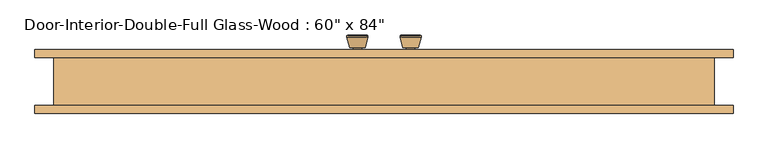
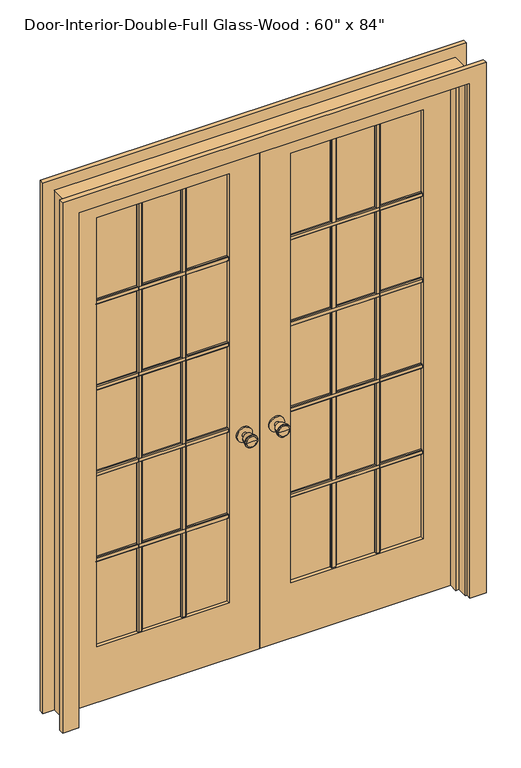
"""IFC4 building model written with IfcOpenShell, lengths in millimetres: door geometry."""

from ifc_helpers import new_model, si_unit, point, frame, frame_2d, origin, place, context, project, spatial, polyline, circle_curve, trimmed, segment, composite_curve, outline, extrude, faceted_brep, source, transform, mapped, element, save
from ifc_brep_helpers import plane_surface, cylinder_surface, revolved_surface, advanced_brep


def door_fac3bb52(model_context):
    return source(origin(), model_context, "Body", "SolidModel", [
        advanced_brep(
        [(-63.5, 59.975, 914.4), (-73.5, 59.975, 914.4), (-53.5, 59.975, 914.4), (-83.9758676, 108.975, 914.4), (-63.5, 108.975, 914.4), (-43.0241324, 108.975, 914.4), (-88.5, 107.1471319, 914.4), (-38.5, 107.1471319, 914.4), (-88.5, 103.6834537, 914.4), (-38.5, 103.6834537, 914.4), (-82.136236, 78.975, 914.4), (-44.863764, 78.975, 914.4), (-73.5, 78.975, 914.4), (-53.5, 78.975, 914.4)],
        [
            (0, 1),
            (1, 2, circle_curve(frame((-63.5, 59.975, 914.4), z_axis=(0.0, -1.0, 0.0), x_axis=(1.0, 0.0, 0.0)), 10.0)),
            (2, 0),
            (2, 1, circle_curve(frame((-63.5, 59.975, 914.4), z_axis=(0.0, -1.0, 0.0), x_axis=(1.0, 0.0, 0.0)), 10.0)),
            (3, 4),
            (4, 5),
            (5, 3, circle_curve(frame((-63.5, 108.975, 914.4), z_axis=(0.0, 1.0, 0.0), x_axis=(1.0, 0.0, 0.0)), 20.4758676)),
            (3, 5, circle_curve(frame((-63.5, 108.975, 914.4), z_axis=(0.0, 1.0, 0.0), x_axis=(1.0, 0.0, 0.0)), 20.4758676)),
            (6, 3),
            (5, 7),
            (7, 6, circle_curve(frame((-63.5, 107.1471319, 914.4), z_axis=(0.0, 1.0, 0.0), x_axis=(1.0, 0.0, 0.0)), 25.0)),
            (6, 7, circle_curve(frame((-63.5, 107.1471319, 914.4), z_axis=(0.0, 1.0, 0.0), x_axis=(1.0, 0.0, 0.0)), 25.0)),
            (8, 6),
            (7, 9),
            (9, 8, circle_curve(frame((-63.5, 103.6834537, 914.4), z_axis=(0.0, 1.0, 0.0), x_axis=(1.0, 0.0, 0.0)), 25.0)),
            (8, 9, circle_curve(frame((-63.5, 103.6834537, 914.4), z_axis=(0.0, 1.0, 0.0), x_axis=(1.0, 0.0, 0.0)), 25.0)),
            (10, 8),
            (9, 11),
            (11, 10, circle_curve(frame((-63.5, 78.975, 914.4), z_axis=(0.0, 1.0, 0.0), x_axis=(1.0, 0.0, 0.0)), 18.636236)),
            (10, 11, circle_curve(frame((-63.5, 78.975, 914.4), z_axis=(0.0, 1.0, 0.0), x_axis=(1.0, 0.0, 0.0)), 18.636236)),
            (12, 10),
            (11, 13),
            (13, 12, circle_curve(frame((-63.5, 78.975, 914.4), z_axis=(0.0, 1.0, 0.0), x_axis=(1.0, 0.0, 0.0)), 10.0)),
            (12, 13, circle_curve(frame((-63.5, 78.975, 914.4), z_axis=(0.0, 1.0, 0.0), x_axis=(1.0, 0.0, 0.0)), 10.0)),
            (1, 12),
            (13, 2),
        ],
        [
            plane_surface(frame((-63.5, 59.975, 914.4), z_axis=(0.0, -1.0, 0.0), x_axis=(1.0, 0.0, 0.0))),
            plane_surface(frame((-63.5, 108.975, 914.4), z_axis=(0.0, 1.0, 0.0), x_axis=(1.0, 0.0, 0.0))),
            revolved_surface(polyline([(-43.0241324, 108.975, 914.4), (-38.5, 107.1471319, 914.4)]), (-63.5, 59.975, 914.4), (0.0, -1.0, 0.0)),
            cylinder_surface(frame((-63.5, 59.975, 914.4), z_axis=(0.0, -1.0, 0.0), x_axis=(1.0, 0.0, 0.0)), 25.0),
            revolved_surface(polyline([(-38.5, 103.6834537, 914.4), (-44.863764, 78.975, 914.4)]), (-63.5, 59.975, 914.4), (0.0, -1.0, 0.0)),
            plane_surface(frame((-63.5, 78.975, 914.4), z_axis=(0.0, -1.0, 0.0), x_axis=(1.0, 0.0, 0.0))),
            cylinder_surface(frame((-63.5, 59.975, 914.4), z_axis=(0.0, -1.0, 0.0), x_axis=(1.0, 0.0, 0.0)), 10.0),
        ],
        [
            (0, [[1, 2, 3]]),
            (0, [[-3, 4, -1]]),
            (1, [[5, 6, 7]]),
            (1, [[-6, -5, 8]]),
            (2, [[9, -7, 10, 11]]),
            (2, [[-10, -8, -9, 12]]),
            (3, [[13, -11, 14, 15]]),
            (3, [[-14, -12, -13, 16]]),
            (4, [[17, -15, 18, 19]]),
            (4, [[-18, -16, -17, 20]]),
            (5, [[21, -19, 22, 23]]),
            (5, [[-22, -20, -21, 24]]),
            (6, [[25, -23, 26, -2]]),
            (6, [[-26, -24, -25, -4]]),
        ],
    ),
        extrude(outline(composite_curve([segment(trimmed(circle_curve(frame_2d((914.4, -63.5)), 30.0), [point((914.4, -33.5))], [point((914.4, -93.5))], False, "CARTESIAN"), True, "CONTINUOUS"), segment(trimmed(circle_curve(frame_2d((914.4, -63.5)), 30.0), [point((914.4, -93.5))], [point((914.4, -33.5))], False, "CARTESIAN"), True, "CONTINUOUS")], self_intersect=False)), frame((0.0, 53.975, 0.0), z_axis=(0.0, 1.0, 0.0), x_axis=(0.0, 0.0, 1.0)), (0.0, 0.0, 1.0), 6.0),
        advanced_brep(
        [(-63.5, 13.05, 914.4), (-53.5, 13.05, 914.4), (-73.5, 13.05, 914.4), (-83.9758676, -35.95, 914.4), (-43.0241324, -35.95, 914.4), (-63.5, -35.95, 914.4), (-88.5, -34.1221319, 914.4), (-38.5, -34.1221319, 914.4), (-88.5, -30.6584537, 914.4), (-38.5, -30.6584537, 914.4), (-82.136236, -5.95, 914.4), (-44.863764, -5.95, 914.4), (-73.5, -5.95, 914.4), (-53.5, -5.95, 914.4)],
        [
            (0, 1),
            (1, 2, circle_curve(frame((-63.5, 13.05, 914.4), z_axis=(0.0, 1.0, 0.0), x_axis=(1.0, 0.0, 0.0)), 10.0)),
            (2, 0),
            (2, 1, circle_curve(frame((-63.5, 13.05, 914.4), z_axis=(0.0, 1.0, 0.0), x_axis=(1.0, 0.0, 0.0)), 10.0)),
            (3, 4, circle_curve(frame((-63.5, -35.95, 914.4), z_axis=(0.0, -1.0, 0.0), x_axis=(1.0, 0.0, 0.0)), 20.4758676)),
            (4, 5),
            (5, 3),
            (4, 3, circle_curve(frame((-63.5, -35.95, 914.4), z_axis=(0.0, -1.0, 0.0), x_axis=(1.0, 0.0, 0.0)), 20.4758676)),
            (6, 7, circle_curve(frame((-63.5, -34.1221319, 914.4), z_axis=(0.0, -1.0, 0.0), x_axis=(1.0, 0.0, 0.0)), 25.0)),
            (7, 4),
            (3, 6),
            (7, 6, circle_curve(frame((-63.5, -34.1221319, 914.4), z_axis=(0.0, -1.0, 0.0), x_axis=(1.0, 0.0, 0.0)), 25.0)),
            (8, 9, circle_curve(frame((-63.5, -30.6584537, 914.4), z_axis=(0.0, -1.0, 0.0), x_axis=(1.0, 0.0, 0.0)), 25.0)),
            (9, 7),
            (6, 8),
            (9, 8, circle_curve(frame((-63.5, -30.6584537, 914.4), z_axis=(0.0, -1.0, 0.0), x_axis=(1.0, 0.0, 0.0)), 25.0)),
            (10, 11, circle_curve(frame((-63.5, -5.95, 914.4), z_axis=(0.0, -1.0, 0.0), x_axis=(1.0, 0.0, 0.0)), 18.636236)),
            (11, 9),
            (8, 10),
            (11, 10, circle_curve(frame((-63.5, -5.95, 914.4), z_axis=(0.0, -1.0, 0.0), x_axis=(1.0, 0.0, 0.0)), 18.636236)),
            (12, 13, circle_curve(frame((-63.5, -5.95, 914.4), z_axis=(0.0, -1.0, 0.0), x_axis=(1.0, 0.0, 0.0)), 10.0)),
            (13, 11),
            (10, 12),
            (13, 12, circle_curve(frame((-63.5, -5.95, 914.4), z_axis=(0.0, -1.0, 0.0), x_axis=(1.0, 0.0, 0.0)), 10.0)),
            (1, 13),
            (12, 2),
        ],
        [
            plane_surface(frame((-63.5, 13.05, 914.4), z_axis=(0.0, 1.0, 0.0), x_axis=(1.0, 0.0, 0.0))),
            plane_surface(frame((-63.5, -35.95, 914.4), z_axis=(0.0, -1.0, 0.0), x_axis=(1.0, 0.0, 0.0))),
            revolved_surface(polyline([(-43.0241324, -35.95, 914.4), (-38.5, -34.1221319, 914.4)]), (-63.5, 13.05, 914.4), (0.0, 1.0, 0.0)),
            cylinder_surface(frame((-63.5, 13.05, 914.4), z_axis=(0.0, 1.0, 0.0), x_axis=(1.0, 0.0, 0.0)), 25.0),
            revolved_surface(polyline([(-38.5, -30.6584537, 914.4), (-44.863764, -5.95, 914.4)]), (-63.5, 13.05, 914.4), (0.0, 1.0, 0.0)),
            plane_surface(frame((-63.5, -5.95, 914.4), z_axis=(0.0, 1.0, 0.0), x_axis=(1.0, 0.0, 0.0))),
            cylinder_surface(frame((-63.5, 13.05, 914.4), z_axis=(0.0, 1.0, 0.0), x_axis=(1.0, 0.0, 0.0)), 10.0),
        ],
        [
            (0, [[1, 2, 3]]),
            (0, [[-3, 4, -1]]),
            (1, [[5, 6, 7]]),
            (1, [[8, -7, -6]]),
            (2, [[9, 10, -5, 11]]),
            (2, [[12, -11, -8, -10]]),
            (3, [[13, 14, -9, 15]]),
            (3, [[16, -15, -12, -14]]),
            (4, [[17, 18, -13, 19]]),
            (4, [[20, -19, -16, -18]]),
            (5, [[21, 22, -17, 23]]),
            (5, [[24, -23, -20, -22]]),
            (6, [[-2, 25, -21, 26]]),
            (6, [[-4, -26, -24, -25]]),
        ],
    ),
        extrude(outline(composite_curve([segment(trimmed(circle_curve(frame_2d((914.4, -63.5)), 30.0), [point((914.4, -33.5))], [point((914.4, -93.5))], False, "CARTESIAN"), True, "CONTINUOUS"), segment(trimmed(circle_curve(frame_2d((914.4, -63.5)), 30.0), [point((914.4, -93.5))], [point((914.4, -33.5))], False, "CARTESIAN"), True, "CONTINUOUS")], self_intersect=False)), frame((0.0, 13.05, 0.0), z_axis=(0.0, 1.0, 0.0), x_axis=(0.0, 0.0, 1.0)), (0.0, 0.0, 1.0), 6.0),
        extrude(outline(polyline([(33.02, 1667.51), (33.02, 1648.46), (26.67, 1648.46), (23.495, 1651.635), (23.495, 1664.335), (26.67, 1667.51), (33.02, 1667.51)])), frame((120.65, 0.0, 0.0), z_axis=(1.0, 0.0, 0.0), x_axis=(0.0, 1.0, 0.0)), (0.0, 0.0, 1.0), 520.7),
        extrude(outline(polyline([(33.02, 1310.9575), (33.02, 1291.9075), (26.67, 1291.9075), (23.495, 1295.0825), (23.495, 1307.7825), (26.67, 1310.9575), (33.02, 1310.9575)])), frame((120.65, 0.0, 0.0), z_axis=(1.0, 0.0, 0.0), x_axis=(0.0, 1.0, 0.0)), (0.0, 0.0, 1.0), 520.7),
        extrude(outline(polyline([(33.02, 954.405), (33.02, 935.355), (26.67, 935.355), (23.495, 938.53), (23.495, 951.23), (26.67, 954.405), (33.02, 954.405)])), frame((120.65, 0.0, 0.0), z_axis=(1.0, 0.0, 0.0), x_axis=(0.0, 1.0, 0.0)), (0.0, 0.0, 1.0), 520.7),
        extrude(outline(polyline([(33.02, 597.8525), (33.02, 578.8025), (26.67, 578.8025), (23.495, 581.9775), (23.495, 594.6775), (26.67, 597.8525), (33.02, 597.8525)])), frame((120.65, 0.0, 0.0), z_axis=(1.0, 0.0, 0.0), x_axis=(0.0, 1.0, 0.0)), (0.0, 0.0, 1.0), 520.7),
        extrude(outline(polyline([(458.2583333, 33.02), (477.3083333, 33.02), (477.3083333, 26.67), (474.1333333, 23.495), (461.4333333, 23.495), (458.2583333, 26.67), (458.2583333, 33.02)])), frame((0.0, 0.0, 231.775), z_axis=(0.0, 0.0, 1.0), x_axis=(1.0, 0.0, 0.0)), (0.0, 0.0, 1.0), 1782.7625),
        extrude(outline(polyline([(284.6916667, 33.02), (303.7416667, 33.02), (303.7416667, 26.67), (300.5666667, 23.495), (287.8666667, 23.495), (284.6916667, 26.67), (284.6916667, 33.02)])), frame((0.0, 0.0, 231.775), z_axis=(0.0, 0.0, 1.0), x_axis=(1.0, 0.0, 0.0)), (0.0, 0.0, 1.0), 1782.7625),
        extrude(outline(polyline([(40.005, 1667.51), (46.355, 1667.51), (49.53, 1664.335), (49.53, 1651.635), (46.355, 1648.46), (40.005, 1648.46), (40.005, 1667.51)])), frame((-641.35, 0.0, 0.0), z_axis=(1.0, 0.0, 0.0), x_axis=(0.0, 1.0, 0.0)), (0.0, 0.0, 1.0), 520.7),
        extrude(outline(polyline([(40.005, 1310.9575), (46.355, 1310.9575), (49.53, 1307.7825), (49.53, 1295.0825), (46.355, 1291.9075), (40.005, 1291.9075), (40.005, 1310.9575)])), frame((-641.35, 0.0, 0.0), z_axis=(1.0, 0.0, 0.0), x_axis=(0.0, 1.0, 0.0)), (0.0, 0.0, 1.0), 520.7),
        extrude(outline(polyline([(40.005, 954.405), (46.355, 954.405), (49.53, 951.23), (49.53, 938.53), (46.355, 935.355), (40.005, 935.355), (40.005, 954.405)])), frame((-641.35, 0.0, 0.0), z_axis=(1.0, 0.0, 0.0), x_axis=(0.0, 1.0, 0.0)), (0.0, 0.0, 1.0), 520.7),
        extrude(outline(polyline([(40.005, 597.8525), (46.355, 597.8525), (49.53, 594.6775), (49.53, 581.9775), (46.355, 578.8025), (40.005, 578.8025), (40.005, 597.8525)])), frame((-641.35, 0.0, 0.0), z_axis=(1.0, 0.0, 0.0), x_axis=(0.0, 1.0, 0.0)), (0.0, 0.0, 1.0), 520.7),
        extrude(outline(polyline([(-303.7416667, 40.005), (-303.7416667, 46.355), (-300.5666667, 49.53), (-287.8666667, 49.53), (-284.6916667, 46.355), (-284.6916667, 40.005), (-303.7416667, 40.005)])), frame((0.0, 0.0, 231.775), z_axis=(0.0, 0.0, 1.0), x_axis=(1.0, 0.0, 0.0)), (0.0, 0.0, 1.0), 1782.7625),
        extrude(outline(polyline([(-477.3083333, 40.005), (-477.3083333, 46.355), (-474.1333333, 49.53), (-461.4333333, 49.53), (-458.2583333, 46.355), (-458.2583333, 40.005), (-477.3083333, 40.005)])), frame((0.0, 0.0, 231.775), z_axis=(0.0, 0.0, 1.0), x_axis=(1.0, 0.0, 0.0)), (0.0, 0.0, 1.0), 1782.7625),
        extrude(outline(polyline([(40.005, 1667.51), (46.355, 1667.51), (49.53, 1664.335), (49.53, 1651.635), (46.355, 1648.46), (40.005, 1648.46), (40.005, 1667.51)])), frame((120.65, 0.0, 0.0), z_axis=(1.0, 0.0, 0.0), x_axis=(0.0, 1.0, 0.0)), (0.0, 0.0, 1.0), 520.7),
        extrude(outline(polyline([(40.005, 1310.9575), (46.355, 1310.9575), (49.53, 1307.7825), (49.53, 1295.0825), (46.355, 1291.9075), (40.005, 1291.9075), (40.005, 1310.9575)])), frame((120.65, 0.0, 0.0), z_axis=(1.0, 0.0, 0.0), x_axis=(0.0, 1.0, 0.0)), (0.0, 0.0, 1.0), 520.7),
        extrude(outline(polyline([(40.005, 954.405), (46.355, 954.405), (49.53, 951.23), (49.53, 938.53), (46.355, 935.355), (40.005, 935.355), (40.005, 954.405)])), frame((120.65, 0.0, 0.0), z_axis=(1.0, 0.0, 0.0), x_axis=(0.0, 1.0, 0.0)), (0.0, 0.0, 1.0), 520.7),
        extrude(outline(polyline([(40.005, 597.8525), (46.355, 597.8525), (49.53, 594.6775), (49.53, 581.9775), (46.355, 578.8025), (40.005, 578.8025), (40.005, 597.8525)])), frame((120.65, 0.0, 0.0), z_axis=(1.0, 0.0, 0.0), x_axis=(0.0, 1.0, 0.0)), (0.0, 0.0, 1.0), 520.7),
        extrude(outline(polyline([(458.2583333, 40.005), (458.2583333, 46.355), (461.4333333, 49.53), (474.1333333, 49.53), (477.3083333, 46.355), (477.3083333, 40.005), (458.2583333, 40.005)])), frame((0.0, 0.0, 231.775), z_axis=(0.0, 0.0, 1.0), x_axis=(1.0, 0.0, 0.0)), (0.0, 0.0, 1.0), 1782.7625),
        extrude(outline(polyline([(284.6916667, 40.005), (284.6916667, 46.355), (287.8666667, 49.53), (300.5666667, 49.53), (303.7416667, 46.355), (303.7416667, 40.005), (284.6916667, 40.005)])), frame((0.0, 0.0, 231.775), z_axis=(0.0, 0.0, 1.0), x_axis=(1.0, 0.0, 0.0)), (0.0, 0.0, 1.0), 1782.7625),
        extrude(outline(polyline([(33.02, 1667.51), (33.02, 1648.46), (26.67, 1648.46), (23.495, 1651.635), (23.495, 1664.335), (26.67, 1667.51), (33.02, 1667.51)])), frame((-641.35, 0.0, 0.0), z_axis=(1.0, 0.0, 0.0), x_axis=(0.0, 1.0, 0.0)), (0.0, 0.0, 1.0), 520.7),
        extrude(outline(polyline([(33.02, 1310.9575), (33.02, 1291.9075), (26.67, 1291.9075), (23.495, 1295.0825), (23.495, 1307.7825), (26.67, 1310.9575), (33.02, 1310.9575)])), frame((-641.35, 0.0, 0.0), z_axis=(1.0, 0.0, 0.0), x_axis=(0.0, 1.0, 0.0)), (0.0, 0.0, 1.0), 520.7),
        extrude(outline(polyline([(33.02, 954.405), (33.02, 935.355), (26.67, 935.355), (23.495, 938.53), (23.495, 951.23), (26.67, 954.405), (33.02, 954.405)])), frame((-641.35, 0.0, 0.0), z_axis=(1.0, 0.0, 0.0), x_axis=(0.0, 1.0, 0.0)), (0.0, 0.0, 1.0), 520.7),
        extrude(outline(polyline([(33.02, 597.8525), (33.02, 578.8025), (26.67, 578.8025), (23.495, 581.9775), (23.495, 594.6775), (26.67, 597.8525), (33.02, 597.8525)])), frame((-641.35, 0.0, 0.0), z_axis=(1.0, 0.0, 0.0), x_axis=(0.0, 1.0, 0.0)), (0.0, 0.0, 1.0), 520.7),
        extrude(outline(polyline([(-303.7416667, 33.02), (-284.6916667, 33.02), (-284.6916667, 26.67), (-287.8666667, 23.495), (-300.5666667, 23.495), (-303.7416667, 26.67), (-303.7416667, 33.02)])), frame((0.0, 0.0, 231.775), z_axis=(0.0, 0.0, 1.0), x_axis=(1.0, 0.0, 0.0)), (0.0, 0.0, 1.0), 1782.7625),
        extrude(outline(polyline([(-477.3083333, 33.02), (-458.2583333, 33.02), (-458.2583333, 26.67), (-461.4333333, 23.495), (-474.1333333, 23.495), (-477.3083333, 26.67), (-477.3083333, 33.02)])), frame((0.0, 0.0, 231.775), z_axis=(0.0, 0.0, 1.0), x_axis=(1.0, 0.0, 0.0)), (0.0, 0.0, 1.0), 1782.7625),
        advanced_brep(
        [(63.5, 13.05, 914.4), (73.5, 13.05, 914.4), (53.5, 13.05, 914.4), (83.9758676, -35.95, 914.4), (63.5, -35.95, 914.4), (43.0241324, -35.95, 914.4), (88.5, -34.1221319, 914.4), (38.5, -34.1221319, 914.4), (88.5, -30.6584537, 914.4), (38.5, -30.6584537, 914.4), (82.136236, -5.95, 914.4), (44.863764, -5.95, 914.4), (73.5, -5.95, 914.4), (53.5, -5.95, 914.4)],
        [
            (0, 1),
            (1, 2, circle_curve(frame((63.5, 13.05, 914.4), z_axis=(0.0, 1.0, 0.0), x_axis=(-1.0, 0.0, 0.0)), 10.0)),
            (2, 0),
            (2, 1, circle_curve(frame((63.5, 13.05, 914.4), z_axis=(0.0, 1.0, 0.0), x_axis=(-1.0, 0.0, 0.0)), 10.0)),
            (3, 4),
            (4, 5),
            (5, 3, circle_curve(frame((63.5, -35.95, 914.4), z_axis=(0.0, -1.0, 0.0), x_axis=(-1.0, 0.0, 0.0)), 20.4758676)),
            (3, 5, circle_curve(frame((63.5, -35.95, 914.4), z_axis=(0.0, -1.0, 0.0), x_axis=(-1.0, 0.0, 0.0)), 20.4758676)),
            (6, 3),
            (5, 7),
            (7, 6, circle_curve(frame((63.5, -34.1221319, 914.4), z_axis=(0.0, -1.0, 0.0), x_axis=(-1.0, 0.0, 0.0)), 25.0)),
            (6, 7, circle_curve(frame((63.5, -34.1221319, 914.4), z_axis=(0.0, -1.0, 0.0), x_axis=(-1.0, 0.0, 0.0)), 25.0)),
            (8, 6),
            (7, 9),
            (9, 8, circle_curve(frame((63.5, -30.6584537, 914.4), z_axis=(0.0, -1.0, 0.0), x_axis=(-1.0, 0.0, 0.0)), 25.0)),
            (8, 9, circle_curve(frame((63.5, -30.6584537, 914.4), z_axis=(0.0, -1.0, 0.0), x_axis=(-1.0, 0.0, 0.0)), 25.0)),
            (10, 8),
            (9, 11),
            (11, 10, circle_curve(frame((63.5, -5.95, 914.4), z_axis=(0.0, -1.0, 0.0), x_axis=(-1.0, 0.0, 0.0)), 18.636236)),
            (10, 11, circle_curve(frame((63.5, -5.95, 914.4), z_axis=(0.0, -1.0, 0.0), x_axis=(-1.0, 0.0, 0.0)), 18.636236)),
            (12, 10),
            (11, 13),
            (13, 12, circle_curve(frame((63.5, -5.95, 914.4), z_axis=(0.0, -1.0, 0.0), x_axis=(-1.0, 0.0, 0.0)), 10.0)),
            (12, 13, circle_curve(frame((63.5, -5.95, 914.4), z_axis=(0.0, -1.0, 0.0), x_axis=(-1.0, 0.0, 0.0)), 10.0)),
            (1, 12),
            (13, 2),
        ],
        [
            plane_surface(frame((63.5, 13.05, 914.4), z_axis=(0.0, 1.0, 0.0), x_axis=(-1.0, 0.0, 0.0))),
            plane_surface(frame((63.5, -35.95, 914.4), z_axis=(0.0, -1.0, 0.0), x_axis=(-1.0, 0.0, 0.0))),
            revolved_surface(polyline([(43.0241324, -35.95, 914.4), (38.5, -34.1221319, 914.4)]), (63.5, 13.05, 914.4), (0.0, 1.0, 0.0)),
            cylinder_surface(frame((63.5, 13.05, 914.4), z_axis=(0.0, 1.0, 0.0), x_axis=(-1.0, 0.0, 0.0)), 25.0),
            revolved_surface(polyline([(38.5, -30.6584537, 914.4), (44.863764, -5.95, 914.4)]), (63.5, 13.05, 914.4), (0.0, 1.0, 0.0)),
            plane_surface(frame((63.5, -5.95, 914.4), z_axis=(0.0, 1.0, 0.0), x_axis=(-1.0, 0.0, 0.0))),
            cylinder_surface(frame((63.5, 13.05, 914.4), z_axis=(0.0, 1.0, 0.0), x_axis=(-1.0, 0.0, 0.0)), 10.0),
        ],
        [
            (0, [[1, 2, 3]]),
            (0, [[-3, 4, -1]]),
            (1, [[5, 6, 7]]),
            (1, [[-6, -5, 8]]),
            (2, [[9, -7, 10, 11]]),
            (2, [[-10, -8, -9, 12]]),
            (3, [[13, -11, 14, 15]]),
            (3, [[-14, -12, -13, 16]]),
            (4, [[17, -15, 18, 19]]),
            (4, [[-18, -16, -17, 20]]),
            (5, [[21, -19, 22, 23]]),
            (5, [[-22, -20, -21, 24]]),
            (6, [[25, -23, 26, -2]]),
            (6, [[-26, -24, -25, -4]]),
        ],
    ),
        extrude(outline(composite_curve([segment(trimmed(circle_curve(frame_2d((914.4, 63.5)), 30.0), [point((914.4, 33.5))], [point((914.4, 93.5))], False, "CARTESIAN"), True, "CONTINUOUS"), segment(trimmed(circle_curve(frame_2d((914.4, 63.5)), 30.0), [point((914.4, 93.5))], [point((914.4, 33.5))], False, "CARTESIAN"), True, "CONTINUOUS")], self_intersect=False)), frame((0.0, 13.05, 0.0), z_axis=(0.0, 1.0, 0.0), x_axis=(0.0, 0.0, 1.0)), (0.0, 0.0, 1.0), 6.0),
        advanced_brep(
        [(63.5, 59.975, 914.4), (53.5, 59.975, 914.4), (73.5, 59.975, 914.4), (83.9758676, 108.975, 914.4), (43.0241324, 108.975, 914.4), (63.5, 108.975, 914.4), (88.5, 107.1471319, 914.4), (38.5, 107.1471319, 914.4), (88.5, 103.6834537, 914.4), (38.5, 103.6834537, 914.4), (82.136236, 78.975, 914.4), (44.863764, 78.975, 914.4), (73.5, 78.975, 914.4), (53.5, 78.975, 914.4)],
        [
            (0, 1),
            (1, 2, circle_curve(frame((63.5, 59.975, 914.4), z_axis=(0.0, -1.0, 0.0), x_axis=(-1.0, 0.0, 0.0)), 10.0)),
            (2, 0),
            (2, 1, circle_curve(frame((63.5, 59.975, 914.4), z_axis=(0.0, -1.0, 0.0), x_axis=(-1.0, 0.0, 0.0)), 10.0)),
            (3, 4, circle_curve(frame((63.5, 108.975, 914.4), z_axis=(0.0, 1.0, 0.0), x_axis=(-1.0, 0.0, 0.0)), 20.4758676)),
            (4, 5),
            (5, 3),
            (4, 3, circle_curve(frame((63.5, 108.975, 914.4), z_axis=(0.0, 1.0, 0.0), x_axis=(-1.0, 0.0, 0.0)), 20.4758676)),
            (6, 7, circle_curve(frame((63.5, 107.1471319, 914.4), z_axis=(0.0, 1.0, 0.0), x_axis=(-1.0, 0.0, 0.0)), 25.0)),
            (7, 4),
            (3, 6),
            (7, 6, circle_curve(frame((63.5, 107.1471319, 914.4), z_axis=(0.0, 1.0, 0.0), x_axis=(-1.0, 0.0, 0.0)), 25.0)),
            (8, 9, circle_curve(frame((63.5, 103.6834537, 914.4), z_axis=(0.0, 1.0, 0.0), x_axis=(-1.0, 0.0, 0.0)), 25.0)),
            (9, 7),
            (6, 8),
            (9, 8, circle_curve(frame((63.5, 103.6834537, 914.4), z_axis=(0.0, 1.0, 0.0), x_axis=(-1.0, 0.0, 0.0)), 25.0)),
            (10, 11, circle_curve(frame((63.5, 78.975, 914.4), z_axis=(0.0, 1.0, 0.0), x_axis=(-1.0, 0.0, 0.0)), 18.636236)),
            (11, 9),
            (8, 10),
            (11, 10, circle_curve(frame((63.5, 78.975, 914.4), z_axis=(0.0, 1.0, 0.0), x_axis=(-1.0, 0.0, 0.0)), 18.636236)),
            (12, 13, circle_curve(frame((63.5, 78.975, 914.4), z_axis=(0.0, 1.0, 0.0), x_axis=(-1.0, 0.0, 0.0)), 10.0)),
            (13, 11),
            (10, 12),
            (13, 12, circle_curve(frame((63.5, 78.975, 914.4), z_axis=(0.0, 1.0, 0.0), x_axis=(-1.0, 0.0, 0.0)), 10.0)),
            (1, 13),
            (12, 2),
        ],
        [
            plane_surface(frame((63.5, 59.975, 914.4), z_axis=(0.0, -1.0, 0.0), x_axis=(-1.0, 0.0, 0.0))),
            plane_surface(frame((63.5, 108.975, 914.4), z_axis=(0.0, 1.0, 0.0), x_axis=(-1.0, 0.0, 0.0))),
            revolved_surface(polyline([(43.0241324, 108.975, 914.4), (38.5, 107.1471319, 914.4)]), (63.5, 59.975, 914.4), (0.0, -1.0, 0.0)),
            cylinder_surface(frame((63.5, 59.975, 914.4), z_axis=(0.0, -1.0, 0.0), x_axis=(-1.0, 0.0, 0.0)), 25.0),
            revolved_surface(polyline([(38.5, 103.6834537, 914.4), (44.863764, 78.975, 914.4)]), (63.5, 59.975, 914.4), (0.0, -1.0, 0.0)),
            plane_surface(frame((63.5, 78.975, 914.4), z_axis=(0.0, -1.0, 0.0), x_axis=(-1.0, 0.0, 0.0))),
            cylinder_surface(frame((63.5, 59.975, 914.4), z_axis=(0.0, -1.0, 0.0), x_axis=(-1.0, 0.0, 0.0)), 10.0),
        ],
        [
            (0, [[1, 2, 3]]),
            (0, [[-3, 4, -1]]),
            (1, [[5, 6, 7]]),
            (1, [[8, -7, -6]]),
            (2, [[9, 10, -5, 11]]),
            (2, [[12, -11, -8, -10]]),
            (3, [[13, 14, -9, 15]]),
            (3, [[16, -15, -12, -14]]),
            (4, [[17, 18, -13, 19]]),
            (4, [[20, -19, -16, -18]]),
            (5, [[21, 22, -17, 23]]),
            (5, [[24, -23, -20, -22]]),
            (6, [[-2, 25, -21, 26]]),
            (6, [[-4, -26, -24, -25]]),
        ],
    ),
        extrude(outline(composite_curve([segment(trimmed(circle_curve(frame_2d((914.4, 63.5)), 30.0), [point((914.4, 33.5))], [point((914.4, 93.5))], False, "CARTESIAN"), True, "CONTINUOUS"), segment(trimmed(circle_curve(frame_2d((914.4, 63.5)), 30.0), [point((914.4, 93.5))], [point((914.4, 33.5))], False, "CARTESIAN"), True, "CONTINUOUS")], self_intersect=False)), frame((0.0, 53.975, 0.0), z_axis=(0.0, 1.0, 0.0), x_axis=(0.0, 0.0, 1.0)), (0.0, 0.0, 1.0), 6.0),
        extrude(outline(polyline([(0.0, 768.35), (0.0, 831.85), (2203.45, 831.85), (2203.45, -831.85), (0.0, -831.85), (0.0, -768.35), (2139.95, -768.35), (2139.95, 768.35), (0.0, 768.35)])), frame((0.0, -79.375, 0.0), z_axis=(0.0, 1.0, 0.0), x_axis=(0.0, 0.0, 1.0)), (0.0, 0.0, 1.0), 19.05),
        extrude(outline(polyline([(0.0, 768.35), (0.0, 831.85), (2203.45, 831.85), (2203.45, -831.85), (0.0, -831.85), (0.0, -768.35), (2139.95, -768.35), (2139.95, 768.35), (0.0, 768.35)])), frame((0.0, 53.975, 0.0), z_axis=(0.0, 1.0, 0.0), x_axis=(0.0, 0.0, 1.0)), (0.0, 0.0, 1.0), 19.05),
        faceted_brep([(787.4, 53.975, 0.0), (787.4, -60.325, 0.0), (762.0, -60.325, 0.0), (762.0, -15.875, 0.0), (749.3, -15.875, 0.0), (749.3, 19.05, 0.0), (762.0, 19.05, 0.0), (762.0, 53.975, 0.0), (787.4, 53.975, 2159.0), (787.4, -60.325, 2159.0), (-787.4, -60.325, 2159.0), (-787.4, -60.325, 0.0), (-762.0, -60.325, 0.0), (-762.0, -60.325, 2133.6), (762.0, -60.325, 2133.6), (762.0, -15.875, 2133.6), (-762.0, -15.875, 2133.6), (-762.0, -15.875, 0.0), (-749.3, -15.875, 0.0), (-749.3, -15.875, 2120.9), (749.3, -15.875, 2120.9), (749.3, 19.05, 2120.9), (1.5875, 19.05, 2120.9), (-1.6019111, 19.05, 2120.9), (-749.3, 19.05, 2120.9), (-749.3, 19.05, 0.0), (-762.0, 19.05, 0.0), (-762.0, 19.05, 2133.6), (-1.6019111, 19.05, 2133.6), (1.5875, 19.05, 2133.6), (762.0, 19.05, 2133.6), (762.0, 53.975, 2133.6), (1.5875, 53.975, 2133.6), (-1.6019111, 53.975, 2133.6), (-762.0, 53.975, 2133.6), (-762.0, 53.975, 0.0), (-787.4, 53.975, 0.0), (-787.4, 53.975, 2159.0)], [[[0, 1, 2, 3, 4, 5, 6, 7]], [[1, 0, 8, 9]], [[2, 1, 9, 10, 11, 12, 13, 14]], [[3, 2, 14, 15]], [[4, 3, 15, 16, 17, 18, 19, 20]], [[5, 4, 20, 21]], [[6, 5, 21, 22, 23, 24, 25, 26, 27, 28, 29, 30]], [[7, 6, 30, 31]], [[0, 7, 31, 32, 33, 34, 35, 36, 37, 8]], [[9, 8, 37, 10]], [[14, 13, 16, 15]], [[20, 19, 24, 23, 22, 21]], [[31, 30, 29, 28, 27, 34, 33, 32]], [[12, 11, 36, 35, 26, 25, 18, 17]], [[11, 10, 37, 36]], [[13, 12, 17, 16]], [[19, 18, 25, 24]], [[27, 26, 35, 34]]]),
        extrude(outline(polyline([(2133.6, -762.0), (0.0, -762.0), (0.0, -1.6019111), (2133.6, -1.6019111), (2133.6, -762.0)]), holes=[polyline([(231.775, -641.35), (2014.5375, -641.35), (2014.5375, -120.65), (231.775, -120.65), (231.775, -641.35)])]), frame((0.0, 19.05, 0.0), z_axis=(0.0, 1.0, 0.0), x_axis=(0.0, 0.0, 1.0)), (0.0, 0.0, 1.0), 34.925),
        extrude(outline(polyline([(0.0, 762.0), (2133.6, 762.0), (2133.6, 1.5875), (0.0, 1.5875), (0.0, 762.0)]), holes=[polyline([(2014.5375, 120.65), (2014.5375, 641.35), (231.775, 641.35), (231.775, 120.65), (2014.5375, 120.65)])]), frame((0.0, 19.05, 0.0), z_axis=(0.0, 1.0, 0.0), x_axis=(0.0, 0.0, 1.0)), (0.0, 0.0, 1.0), 34.925),
        extrude(outline(polyline([(641.35, 33.02), (120.65, 33.02), (120.65, 40.005), (641.35, 40.005), (641.35, 33.02)])), frame((0.0, 0.0, 231.775), z_axis=(0.0, 0.0, 1.0), x_axis=(1.0, 0.0, 0.0)), (0.0, 0.0, 1.0), 1782.7625),
        extrude(outline(polyline([(-120.65, 33.02), (-641.35, 33.02), (-641.35, 40.005), (-120.65, 40.005), (-120.65, 33.02)])), frame((0.0, 0.0, 231.775), z_axis=(0.0, 0.0, 1.0), x_axis=(1.0, 0.0, 0.0)), (0.0, 0.0, 1.0), 1782.7625),
    ])


if __name__ == "__main__":
    model = new_model("IFC4")
    model_context = context("Model", 3, world=origin())
    ifc_project = project(units=[si_unit("LENGTHUNIT", "METRE", prefix="MILLI")], contexts=[model_context])
    site = spatial("IfcSite", under=ifc_project)
    building = spatial("IfcBuilding", under=site)
    placement = place(None, origin())
    door_shape = door_fac3bb52(model_context)
    element("IfcDoor", 1, ObjectType="Door-Interior-Double-Full Glass-Wood : 60\" x 84\"", at=placement, inside=building, context=model_context, shape_type="MappedRepresentation", body=[
        mapped(door_shape, transform((0.0, 0.0, 0.0), x_axis=(1.0, 0.0, 0.0), y_axis=(0.0, 1.0, 0.0), z_axis=(0.0, 0.0, 1.0))),
    ])
    save(model, "model.ifc")

# Revit data of these elements
# Type "Door-Interior-Double-Full Glass-Wood : 60\" x 84\""
#   Type Mark = "9"
#   Assembly Code = "C1020300"
#   Analytic Construction = "French door, wood frame with single glass"
#   Top Rail = 0' - 4 11/16"
#   Thickness = 0' - 1 3/8"
#   Thermal Resistance (R) = 1.0696 (h·ft²·°F)/BTU
#   Swing Angle [instance default] = 90.00°
#   Stiles = 0' - 4 3/4"
#   Rough Width = 5' - 2"
#   Rough Height = 7' - 1"
#   Panel Width = 2' - 6"
#   Height = 7' - 0"
#   Width = 5' - 0"
#   Heat Transfer Coefficient (U) = 0.9350 BTU/(h·ft²·°F)
#   Bottom Rail = 0' - 9 1/8"
#   Show Grill [instance default] = yes
#   Trim Material = Cherry
#   Panel Material = Cherry
#   Frame Material = Cherry
#   Door Handle Material = Aluminum
#   Visual Light Transmittance = 0
#   Solar Heat Gain Coefficient = 0
#   Wall Closure = (empty or 0)
#   Function = (empty or 0)
# Element 1 (IfcDoor, "Door-Interior-Double-Full Glass-Wood : 60\" x 84\"")
#   Materials on its faces: "Cherry", "Aluminum", "Glass"
# Materials
#   "Cherry": class "Wood", colour RGB 226 177 128, transparency 0, Description = "Prunus Serotina", Cost = 0
#   "Aluminum": class "Metal", colour RGB 247 247 247, transparency 0, Description = "Aluminum 6061", Cost = 0
#   "Glass": class "Glass", colour RGB 0 128 192, transparency 0.75, Description = "Soda Lime Glass", Cost = 0
